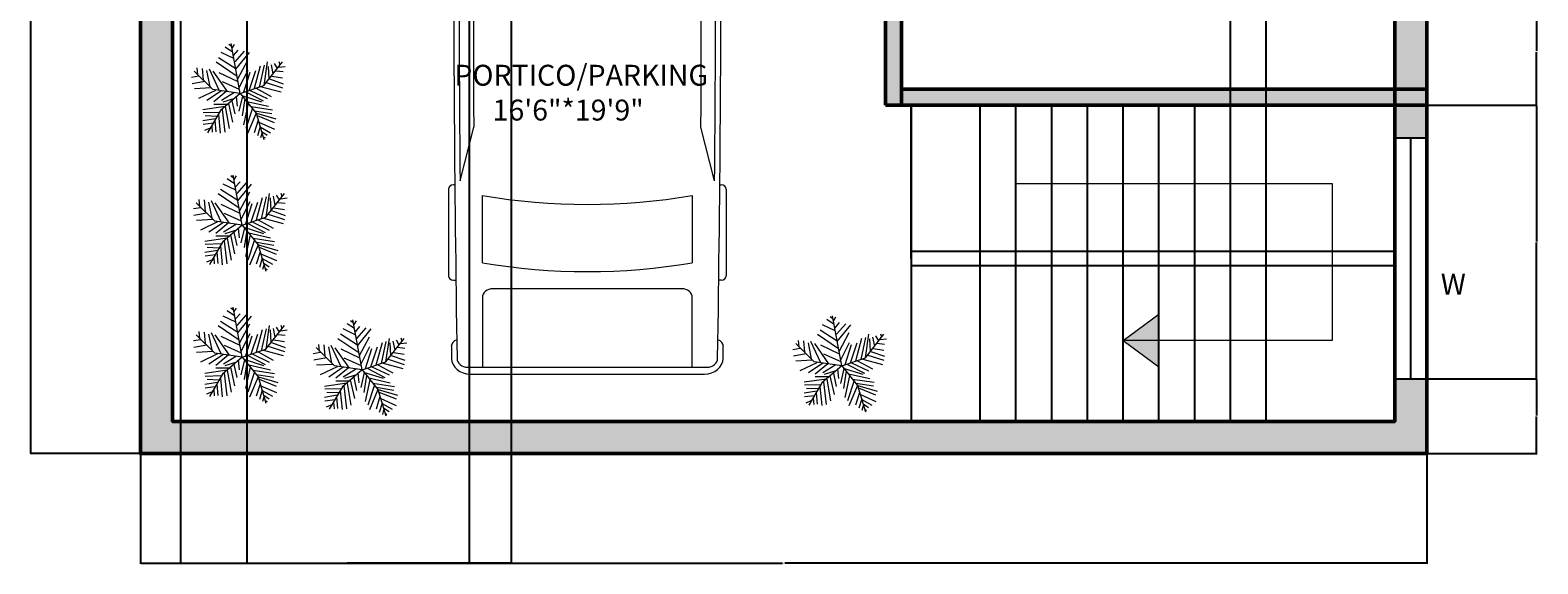
# Model space of a CAD drawing. Units: inches. Extents: x 678 to 1100, y 1432 to 2094.
# Tile 1 of 5: x 678 to 1100, y 1432 to 1581. Entities that reach past the tile are written whole.
import ezdxf

# ---------------------------------------------------------------- set-up
doc = ezdxf.new("R2010")
doc.units = ezdxf.units.IN
for name, color, linetype, lineweight in [('A-ANNO-DIMS', 2, 'Continuous', 18), ('A-ANNO-SYMB', 141, 'Continuous', 18), ('A-AREA-IDEN', 141, 'Continuous', 25), ('A-FLOR-STRS', 8, 'Continuous', 25), ('A-WALL-PATT', 252, 'Continuous', 13), ('C-PRKG-VEHI', 8, 'Continuous', 13), ('TEXT', 141, 'Continuous', 18), ('TREE', 90, 'Continuous', 13), ('WALL', 140, 'Continuous', 50), ('WIND', 212, 'Continuous', 25)]:
    doc.layers.add(name, color=color, linetype=linetype, lineweight=lineweight)
doc.styles.get("Standard").update_dxf_attribs({"font": 'arial.ttf'})
doc.dimstyles.get("Standard").update_dxf_attribs({"dimtxt": 0.18, "dimasz": 0.18, "dimexe": 0.18, "dimexo": 0.0625, "dimgap": 0.09, "dimtad": 0, "dimtih": 1, "dimtoh": 1, "dimdec": 4, "dimzin": 0, "dimdsep": 46, "dimtxsty": 'Standard', "dimcen": 0.09, "dimadec": 0, "dimazin": 0, "dimtfac": 1, "dimtdec": 4, "dimtofl": 0, "dimtmove": 0, "dimatfit": 3, "dimfxl": 1, "dimtolj": 1, "dimtzin": 0, "dimarcsym": 0})

# ---------------------------------------------------------------- blocks, each defined once
blk = doc.blocks.new('*U8')
for p, q in [((46.55, 38.89), (22.35, 38.89)), ((136.7, 38.89), (160.9, 38.89)), ((21.1, 37.41), (21.1, 36.83)), ((47.8, 37.39), (47.8, 37.41)), ((87.99, 31.87), (74.76, 35.92)), ((134.31, 35.6), (119.29, 31.78)), ((135.45, 37.07), (135.45, 37.41)), ((162.15, 37.41), (162.15, 36.77)), ((70.03, 31.54), (86.41, 29.35)), ((186.47, -33.5), (186.47, 33.5)), ((188.4, -32.76), (188.4, 32.76)), ((138.42, 29.35), (157.25, 29.35)), ((164.52, 26.39), (164.52, -26.39)), ((186.47, 29.35), (167.01, 29.35)), ((32.27, 11.63), (36.13, 17.17)), ((36.13, 17.17), (50.94, 17.17)), ((29.77, 9.51), (51.68, 9.51)), ((32.12, 9.51), (32.12, 11.15)), ((58.92, -10.77), (58.92, 10.77)), ((66.55, -10.53), (66.55, 10.53)), ((82.74, 8.5), (82.74, -8.5)), ((186.47, -10.53), (186.47, 10.53)), ((3.27, 6.13), (0.1, 0.41)), ((0, 0), (51.68, 0)), ((0.1, -0.41), (3.27, -6.13)), ((29.77, -9.51), (51.68, -9.51)), ((32.12, -9.51), (32.12, -11.15)), ((32.27, -11.63), (36.13, -17.17)), ((36.13, -17.17), (50.94, -17.17)), ((86.41, -29.35), (70.03, -31.54)), ((157.25, -29.35), (138.42, -29.35)), ((167.01, -29.35), (186.47, -29.35)), ((87.99, -31.87), (74.76, -35.92)), ((134.31, -35.6), (119.29, -31.78)), ((21.1, -37.41), (21.1, -36.83)), ((47.8, -37.39), (47.8, -37.41)), ((135.45, -37.07), (135.45, -37.41)), ((162.15, -37.41), (162.15, -36.77)), ((46.55, -38.89), (22.35, -38.89)), ((136.7, -38.89), (160.9, -38.89))]:
    blk.add_line(p, q)
for centre, major_axis, ratio, start_param, end_param in [((22.35, 37.41), (0, -1.48), 0.842304, 3.141593, 4.712389), ((46.55, 37.41), (0, 1.48), 0.842304, -1.570796, 0), ((136.7, 37.41), (0, -1.48), 0.842304, 3.141593, 4.712389), ((160.9, 37.41), (0, 1.48), 0.842304, -1.570796, 0), ((180.63, 35.84), (0, 2.22), 0.842304, -0.013017, 1.249894), ((64.48, -10556.36), (0, 10595.31), 0.842304, -0.013397, -0.013017), ((183.98, 32.76), (0, -5.25), 0.842304, 1.570796, 3.128196), ((266.03, -27.52), (0, 313.31), 0.842304, 1.367076, 1.39176), ((41.19, -490.86), (0, 528.23), 0.842304, 0.00281, 0.075598), ((64.48, -10555.62), (0, 10593.03), 0.842304, -0.013397, 0.002797), ((64.48, -10555.62), (0, -10591.55), 0.842304, 3.133765, 3.140441), ((183.98, 33.5), (0, -2.96), 0.842304, 1.570796, 3.128196), ((37.47, -593.96), (0, -623.33), 0.842304, 3.096046, 3.200911), ((135.29, 5.39), (0, 81.77), 0.842304, 1.245306, 1.50788), ((95.79, -3666.35), (0, -3698.24), 0.842304, 3.134049, 3.144098), ((259.18, -27.52), (0, -305.3), 0.842304, 4.528606, 4.561838), ((134.4, 5.39), (0, -89.78), 0.842304, 4.449482, 4.652344), ((149.6, 2.8), (0, -79.58), 0.842304, 4.372215, 4.640744), ((17.08, 0), (0, 147.02), 0.842304, 4.511394, 4.913384), ((35.91, 0), (0, 147.02), 0.842304, 4.511394, 4.913384), ((167.01, 26.39), (0, 2.96), 0.842304, 0, 1.570796), ((-204.49, 52.4), (0, -250.96), 0.842304, 1.385369, 1.434372), ((13.04, 17.01), (0, 27.42), 0.842304, 4.435146, 4.718221), ((14.2, 17.01), (0, 27.42), 0.842304, 4.435146, 4.718221), ((50.79, 13.34), (6.34, -0.36), 0.603834, -1.395552, 1.581315), ((29.77, -46.66), (0, 56.17), 0.842304, 0, 0.590319), ((32.75, 11.15), (0, 0.74), 0.842304, 0.879714, 1.570796), ((0.62, 0), (0, -0.74), 0.842304, 4.131459, 5.293319), ((29.77, 46.66), (0, 56.17), 0.842304, 2.551274, 3.141593), ((-204.49, -52.4), (0, 250.96), 0.842304, -1.434372, -1.385369), ((32.75, -11.15), (0, -0.74), 0.842304, 4.712389, 5.403472), ((13.04, -17.01), (0, -27.42), 0.842304, 1.564964, 1.848039), ((14.2, -17.01), (0, -27.42), 0.842304, 1.564964, 1.848039), ((134.4, -5.39), (0, -89.78), 0.842304, -1.510751, -1.307889), ((135.29, -5.39), (0, -81.77), 0.842304, -1.50788, -1.245306), ((149.6, -2.8), (0, -79.58), 0.842304, -1.499151, -1.230623), ((259.18, 27.52), (0, 305.3), 0.842304, 1.721348, 1.754579), ((266.03, 27.52), (0, 313.31), 0.842304, 1.749832, 1.774517), ((37.47, 593.96), (0, -623.33), 0.842304, -0.059319, 0.045547), ((167.01, -26.39), (0, -2.96), 0.842304, 4.712389, 6.283185), ((95.79, 3666.35), (0, -3698.24), 0.842304, -0.002505, 0.007544), ((183.98, -33.5), (0, 2.96), 0.842304, 3.15499, 4.712389), ((183.98, -32.76), (0, -5.25), 0.842304, 0.013397, 1.570796), ((41.19, 490.86), (0, -528.23), 0.842304, -0.075598, -0.00281), ((22.35, -37.41), (0, 1.48), 0.842304, 1.570796, 3.141593), ((64.48, 10555.62), (0, 10593.03), 0.842304, 3.138796, 3.15499), ((46.55, -37.41), (0, -1.48), 0.842304, 0, 1.570796), ((64.48, 10555.62), (0, -10591.55), 0.842304, 0.001152, 0.007828), ((136.7, -37.41), (0, -1.48), 0.842304, -1.570796, 0), ((160.9, -37.41), (0, 1.48), 0.842304, 3.141593, 4.712389), ((180.63, -35.84), (0, -2.22), 0.842304, -1.249894, 0.013017), ((64.48, 10556.36), (0, 10595.31), 0.842304, 3.15461, 3.15499)]:
    blk.add_ellipse(centre, major_axis=major_axis, ratio=ratio, start_param=start_param, end_param=end_param)
at = {"extrusion": (0, 0, -1)}
blk.add_ellipse((50.79, -13.34), major_axis=(6.34, 0.36), ratio=0.603834, start_param=-1.395552, end_param=1.581315, dxfattribs=at)
blk = doc.blocks.new('*U6')
for p, q in [((-8.737, 47.138), (-17.069, 52.711)), ((-10.186, 53.64), (-13.084, 55.962)), ((0, 0), (-10.5, 57)), ((-9.099, 51.782), (-6.563, 55.962)), ((-3.665, 19.273), (-27.574, 35.527)), ((-5.114, 28.097), (-24.676, 40.636)), ((-7.288, 39.707), (-21.778, 46.673)), ((-7.65, 43.423), (-2.578, 49.46)), ((-5.839, 35.992), (4.667, 48.067)), ((-5.114, 27.632), (10.463, 46.673)), ((-2.941, 16.486), (8.652, 37.85)), ((27, 9), (48, 36)), ((27.127, 9.056), (31.112, 35.992)), ((44.153, 36.456), (45.239, 32.741)), ((-47.498, 19.737), (-55.83, 18.344)), ((-31.5, 4.5), (-52.5, 25.5)), ((-48.585, 21.131), (-49.309, 29.026)), ((-43.513, 28.561), (-42.427, 15.558)), ((-38.442, 26.239), (-34.819, 7.663)), ((-35.544, 28.097), (-24.314, 3.947)), ((-14.533, 2.09), (-30.834, 25.31)), ((-24.314, 23.917), (-2.941, 13.7)), ((-1.129, 6.734), (9.014, 26.704)), ((3.942, 1.625), (11.187, 24.381)), ((10.101, 3.483), (17.708, 26.239)), ((16.259, 5.805), (23.142, 31.348)), ((22.055, 7.198), (27.489, 32.277)), ((31.836, 30.883), (32.561, 16.486)), ((35.096, 32.741), (37.27, 22.524)), ((36.183, 19.737), (48.137, 17.88)), ((38.719, 34.134), (41.979, 28.561)), ((40.53, 25.775), (48.862, 24.846)), ((43.791, 29.954), (51.036, 30.883)), ((-40.615, 13.7), (-55.105, 10.913)), ((-33.37, 6.269), (-52.207, 5.34)), ((-28.299, 3.483), (-47.86, -5.805)), ((-21.416, 3.018), (-38.079, -8.128)), ((0, 0), (-31.5, 4.5)), ((-15.982, 2.09), (-30.11, -9.521)), ((0, 0), (-22.5, -19.5)), ((-6.563, 1.161), (-21.416, -8.128)), ((-20.691, 13.7), (-1.129, 4.876)), ((0, 0), (27, 9)), ((0, 0), (18, -22.5)), ((6.478, 1.625), (26.04, -8.592)), ((11.187, 3.483), (30.749, -5.805)), ((18.07, 5.805), (35.096, -3.483)), ((24.229, 7.663), (46.688, 1.625)), ((29.662, 12.307), (48.137, 6.269)), ((33.285, 16.486), (48.862, 10.913)), ((-17.431, -15.094), (-42.789, -18.809)), ((-15.257, -12.772), (-30.11, -12.772)), ((-6.563, -5.805), (-19.967, -9.985)), ((-17.069, -15.094), (-12.721, -40.172)), ((-13.446, -11.378), (-8.737, -32.741)), ((-9.461, -8.592), (-6.201, -23.453)), ((-4.752, -3.483), (-3.665, -14.629)), ((2.493, -3.019), (-1.491, -20.202)), ((1.769, -2.555), (24.229, -9.521)), ((5.029, -6.27), (2.131, -25.775)), ((9.014, -11.378), (3.58, -35.992)), ((14.085, -16.951), (6.478, -40.172)), ((7.565, -9.056), (32.198, -14.629)), ((12.274, -15.094), (36.907, -18.809)), ((-28.299, -29.026), (-42.789, -31.348)), ((-24.314, -21.596), (-42.427, -22.06)), ((-30.834, -34.135), (-42.427, -35.528)), ((-26.849, -26.24), (-40.253, -25.775)), ((-22.5, -19.5), (-37.5, -45)), ((-29.023, -30.884), (-27.936, -43.887)), ((-25.038, -23.918), (-22.865, -45.281)), ((-20.691, -18.345), (-17.793, -44.352)), ((18.07, -22.524), (8.289, -45.745)), ((20.244, -30.419), (15.897, -44.816)), ((16.259, -19.738), (36.183, -22.989)), ((18, -22.5), (27, -52.5)), ((18.433, -22.524), (40.53, -29.026)), ((19.157, -25.311), (38.719, -33.206)), ((21.331, -32.741), (39.081, -40.636)), ((-34.457, -39.708), (-40.978, -42.494)), ((-32.646, -36.921), (-31.921, -44.352)), ((22.78, -37.85), (19.519, -48.532)), ((22.78, -38.314), (34.372, -44.816)), ((24.591, -45.745), (23.142, -50.854)), ((24.591, -43.423), (30.749, -47.603)), ((26.764, -49.925), (28.213, -50.854))]:
    blk.add_line(p, q)
blk = doc.blocks.new('WIN-STANDARD')
blk.add_line((4.5, 0), (4.5, 67.31))
blk.add_lwpolyline([(9, 67.31), (0, 67.31), (0, 0), (9, 0)], close=True)
blk = doc.blocks.new('*D24')
at = {"layer": 'A-ANNO-DIMS', "color": 0, "lineweight": -2, "transparency": 16777216}
for p, q in [((708.96, 1462.87), (708.96, 1432.1)), ((1068.96, 1462.87), (1068.96, 1432.1)), ((709.14, 1432.28), (888.67, 1432.28)), ((1068.78, 1432.28), (889.25, 1432.28))]:
    blk.add_line(p, q, dxfattribs=at)
at = {"layer": 'A-ANNO-DIMS', "color": 0, "transparency": 16777216}
for points in [[(709.14, 1432.31), (709.14, 1432.25), (708.96, 1432.28)], [(1068.78, 1432.31), (1068.78, 1432.25), (1068.96, 1432.28)]]:
    blk.add_solid(points, dxfattribs=at)
at = {"layer": 'Defpoints', "color": 0, "transparency": 16777216}
for p in [(708.96, 1462.93), (1068.96, 1462.93), (1068.96, 1432.28)]:
    blk.add_point(p, dxfattribs=at)
at = {"layer": 'A-ANNO-DIMS', "color": 0, "transparency": 16777216, "insert": (888.96, 1432.28), "char_height": 0.18, "attachment_point": 5}
blk.add_mtext('\\A1;360', dxfattribs=at)
blk = doc.blocks.new('*D25')
at = {"layer": 'A-ANNO-DIMS', "color": 0, "lineweight": -2, "transparency": 16777216}
for p, q in [((708.9, 2062.93), (678.13, 2062.93)), ((678.31, 2062.75), (678.31, 1763.11)), ((678.31, 1463.11), (678.31, 1762.75)), ((708.9, 1462.93), (678.13, 1462.93))]:
    blk.add_line(p, q, dxfattribs=at)
at = {"layer": 'A-ANNO-DIMS', "color": 0, "transparency": 16777216}
for points in [[(678.28, 2062.75), (678.34, 2062.75), (678.31, 2062.93)], [(678.28, 1463.11), (678.34, 1463.11), (678.31, 1462.93)]]:
    blk.add_solid(points, dxfattribs=at)
at = {"layer": 'Defpoints', "color": 0, "transparency": 16777216}
for p in [(678.31, 2062.93), (708.96, 2062.93), (708.96, 1462.93)]:
    blk.add_point(p, dxfattribs=at)
at = {"layer": 'A-ANNO-DIMS', "color": 0, "transparency": 16777216, "insert": (678.31, 1762.93), "char_height": 0.18, "attachment_point": 5}
blk.add_mtext('\\A1;600', dxfattribs=at)
blk = doc.blocks.new('*D31')
at = {"layer": 'A-ANNO-DIMS', "color": 0, "lineweight": -2, "transparency": 16777216}
for p, q in [((1069.02, 1483.85), (1099.79, 1483.85)), ((1099.61, 1483.67), (1099.61, 1473.57)), ((1099.61, 1463.11), (1099.61, 1473.21)), ((1069.02, 1462.93), (1099.79, 1462.93))]:
    blk.add_line(p, q, dxfattribs=at)
at = {"layer": 'A-ANNO-DIMS', "color": 0, "transparency": 16777216}
for points in [[(1099.58, 1483.67), (1099.64, 1483.67), (1099.61, 1483.85)], [(1099.58, 1463.11), (1099.64, 1463.11), (1099.61, 1462.93)]]:
    blk.add_solid(points, dxfattribs=at)
at = {"layer": 'Defpoints', "color": 0, "transparency": 16777216}
for p in [(1068.96, 1483.85), (1099.61, 1483.85), (1068.96, 1462.93)]:
    blk.add_point(p, dxfattribs=at)
at = {"layer": 'A-ANNO-DIMS', "color": 0, "transparency": 16777216, "insert": (1099.61, 1473.39), "char_height": 0.18, "attachment_point": 5}
blk.add_mtext('\\A1;20.922', dxfattribs=at)
blk = doc.blocks.new('*D32')
at = {"layer": 'A-ANNO-DIMS', "color": 0, "lineweight": -2, "transparency": 16777216}
for p, q in [((1069.02, 1560.43), (1099.79, 1560.43)), ((1099.61, 1560.25), (1099.61, 1522.32)), ((1099.61, 1484.03), (1099.61, 1521.96)), ((1069.02, 1483.85), (1099.79, 1483.85))]:
    blk.add_line(p, q, dxfattribs=at)
at = {"layer": 'A-ANNO-DIMS', "color": 0, "transparency": 16777216}
for points in [[(1099.58, 1560.25), (1099.64, 1560.25), (1099.61, 1560.43)], [(1099.58, 1484.03), (1099.64, 1484.03), (1099.61, 1483.85)]]:
    blk.add_solid(points, dxfattribs=at)
at = {"layer": 'Defpoints', "color": 0, "transparency": 16777216}
for p in [(1068.96, 1560.43), (1099.61, 1560.43), (1068.96, 1483.85)]:
    blk.add_point(p, dxfattribs=at)
at = {"layer": 'A-ANNO-DIMS', "color": 0, "transparency": 16777216, "insert": (1099.61, 1522.14), "char_height": 0.18, "attachment_point": 5}
blk.add_mtext('\\A1;76.58', dxfattribs=at)
blk = doc.blocks.new('*D33')
at = {"layer": 'A-ANNO-DIMS', "color": 0, "lineweight": -2, "transparency": 16777216}
for p, q in [((1069.02, 1590.39), (1099.79, 1590.39)), ((1099.61, 1590.21), (1099.61, 1575.59)), ((1099.61, 1560.61), (1099.61, 1575.23)), ((1069.02, 1560.43), (1099.79, 1560.43))]:
    blk.add_line(p, q, dxfattribs=at)
at = {"layer": 'A-ANNO-DIMS', "color": 0, "transparency": 16777216}
for points in [[(1099.58, 1590.21), (1099.64, 1590.21), (1099.61, 1590.39)], [(1099.58, 1560.61), (1099.64, 1560.61), (1099.61, 1560.43)]]:
    blk.add_solid(points, dxfattribs=at)
at = {"layer": 'Defpoints', "color": 0, "transparency": 16777216}
for p in [(1068.96, 1590.39), (1099.61, 1590.39), (1068.96, 1560.43)]:
    blk.add_point(p, dxfattribs=at)
at = {"layer": 'A-ANNO-DIMS', "color": 0, "transparency": 16777216, "insert": (1099.61, 1575.41), "char_height": 0.18, "attachment_point": 5}
blk.add_mtext('\\A1;29.96', dxfattribs=at)
blk = doc.blocks.new('*D48')
at = {"layer": 'A-ANNO-DIMS', "color": 0, "lineweight": -2, "transparency": 16777216}
for p, q in [((917.46, 1560.49), (917.46, 2093.76)), ((917.64, 2093.58), (919.45, 2093.58)), ((921.78, 2093.58), (919.97, 2093.58)), ((921.96, 1560.49), (921.96, 2093.76))]:
    blk.add_line(p, q, dxfattribs=at)
at = {"layer": 'A-ANNO-DIMS', "color": 0, "transparency": 16777216}
for points in [[(917.64, 2093.61), (917.64, 2093.55), (917.46, 2093.58)], [(921.78, 2093.61), (921.78, 2093.55), (921.96, 2093.58)]]:
    blk.add_solid(points, dxfattribs=at)
at = {"layer": 'Defpoints', "color": 0, "transparency": 16777216}
for p in [(921.96, 2093.58), (917.46, 1560.43), (921.96, 1560.43)]:
    blk.add_point(p, dxfattribs=at)
at = {"layer": 'A-ANNO-DIMS', "color": 0, "transparency": 16777216, "insert": (919.71, 2093.58), "char_height": 0.18, "attachment_point": 5}
blk.add_mtext('\\A1;4.5', dxfattribs=at)
blk = doc.blocks.new('*D49')
at = {"layer": 'A-ANNO-DIMS', "color": 0, "lineweight": -2, "transparency": 16777216}
for p, q in [((1013.96, 1471.99), (1013.96, 2093.76)), ((1014.14, 2093.58), (1018.75, 2093.58)), ((1023.78, 2093.58), (1019.17, 2093.58)), ((1023.96, 1471.99), (1023.96, 2093.76))]:
    blk.add_line(p, q, dxfattribs=at)
at = {"layer": 'A-ANNO-DIMS', "color": 0, "transparency": 16777216}
for points in [[(1014.14, 2093.61), (1014.14, 2093.55), (1013.96, 2093.58)], [(1023.78, 2093.61), (1023.78, 2093.55), (1023.96, 2093.58)]]:
    blk.add_solid(points, dxfattribs=at)
at = {"layer": 'Defpoints', "color": 0, "transparency": 16777216}
for p in [(1023.96, 2093.58), (1013.96, 1471.93), (1023.96, 1471.93)]:
    blk.add_point(p, dxfattribs=at)
at = {"layer": 'A-ANNO-DIMS', "color": 0, "transparency": 16777216, "insert": (1018.96, 2093.58), "char_height": 0.18, "attachment_point": 5}
blk.add_mtext('\\A1;10', dxfattribs=at)
blk = doc.blocks.new('*D50')
at = {"layer": 'A-ANNO-DIMS', "color": 0, "lineweight": -2, "transparency": 16777216}
for p, q in [((1023.96, 1471.99), (1023.96, 2093.76)), ((1024.14, 2093.58), (1041.74, 2093.58)), ((1059.78, 2093.58), (1042.18, 2093.58)), ((1059.96, 1471.99), (1059.96, 2093.76))]:
    blk.add_line(p, q, dxfattribs=at)
at = {"layer": 'A-ANNO-DIMS', "color": 0, "transparency": 16777216}
for points in [[(1024.14, 2093.61), (1024.14, 2093.55), (1023.96, 2093.58)], [(1059.78, 2093.61), (1059.78, 2093.55), (1059.96, 2093.58)]]:
    blk.add_solid(points, dxfattribs=at)
at = {"layer": 'Defpoints', "color": 0, "transparency": 16777216}
for p in [(1059.96, 2093.58), (1023.96, 1471.93), (1059.96, 1471.93)]:
    blk.add_point(p, dxfattribs=at)
at = {"layer": 'A-ANNO-DIMS', "color": 0, "transparency": 16777216, "insert": (1041.96, 2093.58), "char_height": 0.18, "attachment_point": 5}
blk.add_mtext('\\A1;36', dxfattribs=at)
blk = doc.blocks.new('*D53')
at = {"layer": 'A-ANNO-DIMS', "color": 0, "lineweight": -2, "transparency": 16777216}
for p, q in [((738.71, 1897.06), (738.71, 1432.1)), ((800.95, 1897.06), (800.95, 1432.1)), ((738.89, 1432.28), (769.43, 1432.28)), ((800.77, 1432.28), (770.22, 1432.28))]:
    blk.add_line(p, q, dxfattribs=at)
at = {"layer": 'A-ANNO-DIMS', "color": 0, "transparency": 16777216}
for points in [[(738.89, 1432.31), (738.89, 1432.25), (738.71, 1432.28)], [(800.77, 1432.31), (800.77, 1432.25), (800.95, 1432.28)]]:
    blk.add_solid(points, dxfattribs=at)
at = {"layer": 'Defpoints', "color": 0, "transparency": 16777216}
for p in [(738.71, 1897.12), (800.95, 1897.12), (800.95, 1432.28)]:
    blk.add_point(p, dxfattribs=at)
at = {"layer": 'A-ANNO-DIMS', "color": 0, "transparency": 16777216, "insert": (769.83, 1432.28), "char_height": 0.18, "attachment_point": 5}
blk.add_mtext('\\A1;62.25', dxfattribs=at)
blk = doc.blocks.new('*D55')
at = {"layer": 'A-ANNO-DIMS', "color": 0, "lineweight": -2, "transparency": 16777216}
for p, q in [((812.72, 1833.21), (812.72, 1432.1)), ((720.22, 1787.87), (720.22, 1432.1)), ((720.4, 1432.28), (766.15, 1432.28)), ((812.54, 1432.28), (766.8, 1432.28))]:
    blk.add_line(p, q, dxfattribs=at)
at = {"layer": 'A-ANNO-DIMS', "color": 0, "transparency": 16777216}
for points in [[(720.4, 1432.31), (720.4, 1432.25), (720.22, 1432.28)], [(812.54, 1432.31), (812.54, 1432.25), (812.72, 1432.28)]]:
    blk.add_solid(points, dxfattribs=at)
at = {"layer": 'Defpoints', "color": 0, "transparency": 16777216}
for p in [(812.72, 1833.27), (720.22, 1787.94), (812.72, 1432.28)]:
    blk.add_point(p, dxfattribs=at)
at = {"layer": 'A-ANNO-DIMS', "color": 0, "transparency": 16777216, "insert": (766.47, 1432.28), "char_height": 0.18, "attachment_point": 5}
blk.add_mtext('\\A1;92.5', dxfattribs=at)

msp = doc.modelspace()

# ---------------------------------------------------------------- hatches: boundary and pattern name
at = {"layer": 'A-ANNO-SYMB'}
h = msp.add_hatch(color=256, dxfattribs=at)
h.dxf.hatch_style = 1
h.paths.add_polyline_path([(993.9606, 1501.9868), (983.9606, 1494.6187), (993.9606, 1494.6187)])
h.paths.add_polyline_path([(993.9606, 1494.6187), (983.9606, 1494.6187), (993.9606, 1487.2506)])
at = {"layer": 'A-WALL-PATT'}
h = msp.add_hatch(color=256, dxfattribs=at)
h.dxf.hatch_style = 1
h.paths.add_polyline_path([(859.7133, 2062.9286), (708.9606, 2062.9286), (708.9606, 2031.3203), (717.9606, 2031.3203), (717.9606, 2053.9286), (837.9606, 2053.9286), (859.7133, 2053.9286)])
h.paths.add_polyline_path([(957.0069, 2062.9286), (896.0724, 2062.9286), (896.0724, 2053.9286), (957.0069, 2053.9286)])
h.paths.add_polyline_path([(842.4606, 2053.9286), (837.9606, 2053.9286), (837.9606, 2005.4286), (842.4606, 2005.4286), (923.4606, 2005.4286), (923.4606, 2009.9286), (842.4606, 2009.9286)])
h.paths.add_polyline_path([(927.9606, 2053.9286), (923.4606, 2053.9286), (923.4606, 2052.1286), (924.8103, 2052.1286), (927.9606, 2052.1286)])
h.paths.add_polyline_path([(1068.9606, 2062.9286), (1024.3184, 2062.9286), (1024.3184, 2053.9286), (1028.6041, 2053.9286), (1059.9606, 2053.9286), (1059.9606, 2002.6361), (1068.9606, 2002.6361)])
h.paths.add_polyline_path([(1059.9606, 1861.9286), (996.9604, 1861.9286), (927.9606, 1861.9286), (923.4606, 1861.9286), (923.4606, 1857.4286), (1059.9606, 1857.4286)], flags=17)
h.paths.add_polyline_path([(927.9606, 2031.1269), (924.8103, 2031.1269, -0.01607952), (923.4606, 2031.1703), (923.4606, 1905.3856), (927.9606, 1905.3856)])
h.paths.add_polyline_path([(923.4606, 1957.9286), (842.4606, 1957.9286), (842.4606, 1969.339), (837.9606, 1969.339), (837.9606, 1953.4286), (923.4606, 1953.4286)])
h.paths.add_polyline_path([(774.6357, 1957.9286), (717.9606, 1957.9286), (717.9606, 1953.4286), (774.6357, 1953.4286)])
h.paths.add_polyline_path([(717.9606, 1979.9404), (708.9606, 1979.9404), (708.9606, 1945.1463), (717.9606, 1945.1463)])
h.paths.add_polyline_path([(840.5596, 1861.9286), (717.9606, 1861.9286), (717.9606, 1857.4286), (840.5596, 1857.4286)], flags=17)
h.paths.add_polyline_path([(927.9606, 1865.3856), (923.4606, 1865.3856), (923.4606, 1861.9286), (927.9606, 1861.9286)], flags=17)
h.paths.add_polyline_path([(1059.9606, 1689.4286), (967.3461, 1689.4286), (967.3461, 1684.9286), (1059.9606, 1684.9286)], flags=17)
h.paths.add_polyline_path([(987.9606, 1737.4286), (983.4606, 1737.4286), (983.4606, 1715.196), (986.7357, 1715.196, -0.01403382), (987.9606, 1715.1616)], flags=17)
h.paths.add_polyline_path([(916.0499, 2036.8414), (924.8721, 2036.8414), (924.8721, 2048.8901), (916.0499, 2048.8901)], flags=9)
h.paths.add_polyline_path([(921.7778, 1883.2914), (930.5999, 1883.2914), (930.5999, 1895.3401), (921.7778, 1895.3401)], flags=25)
h.paths.add_polyline_path([(732.1085, 1683.0506), (740.9307, 1683.0506), (740.9307, 1695.0993), (732.1085, 1695.0993)], flags=25)
h.paths.add_polyline_path([(943.8458, 1737.5114), (952.6679, 1737.5114), (952.6679, 1749.5601), (943.8458, 1749.5601)], flags=25)
h.paths.add_polyline_path([(986.0751, 1696.9795), (994.8973, 1696.9795), (994.8973, 1709.0282), (986.0751, 1709.0282)], flags=25)
h.paths.add_polyline_path([(940.1881, 1677.378), (949.0103, 1677.378), (949.0103, 1689.4267), (940.1881, 1689.4267)], flags=25)
h.paths.add_polyline_path([(998.6262, 1761.7469), (1044.0453, 1761.7469), (1044.0453, 1783.5644), (998.6262, 1783.5644)], flags=25)
h.paths.add_polyline_path([(997.3001, 1713.4735), (1028.9316, 1713.4735), (1028.9316, 1735.2909), (997.3001, 1735.2909)], flags=25)
h.paths.add_polyline_path([(1005.9896, 1586.8139), (1051.4087, 1586.8139), (1051.4087, 1608.6313), (1005.9896, 1608.6313)], flags=25)
h.paths.add_polyline_path([(794.7038, 1552.8124), (873.8721, 1552.8124), (873.8721, 1574.6298), (794.7038, 1574.6298)], flags=25)
h.paths.add_polyline_path([(774.2693, 1771.1228), (831.9444, 1771.1228), (831.9444, 1792.9403), (774.2693, 1792.9403)], flags=25)
h.paths.add_polyline_path([(750.0357, 1897.1514), (786.4291, 1897.1514), (786.4291, 1918.9689), (750.0357, 1918.9689)], flags=25)
h.paths.add_polyline_path([(974.9086, 1953.7921), (1020.3276, 1953.7921), (1020.3276, 1975.6096), (974.9086, 1975.6096)], flags=9)
h.paths.add_polyline_path([(859.1564, 1973.8092), (890.2175, 1973.8092), (890.2175, 1995.6267), (859.1564, 1995.6267)], flags=9)
h.paths.add_polyline_path([(753.2305, 1989.0219), (792.2962, 1989.0219), (792.2962, 2010.8393), (753.2305, 2010.8393)], flags=9)
h.paths.add_polyline_path([(1067.3992, 1620.1515), (1078.032, 1620.1515), (1078.032, 1632.2002), (1067.3992, 1632.2002)], flags=9)
h.paths.add_polyline_path([(846.8446, 2028.8178), (878.5079, 2028.8178), (878.5079, 2050.6353), (846.8446, 2050.6353)], flags=25)
h.paths.add_polyline_path([(1059.9606, 1832.7202), (1068.9606, 1832.7202), (1068.9606, 1935.3246), (1059.9606, 1935.3246)])
h.paths.add_polyline_path([(1068.9606, 1765.4088), (1059.9606, 1765.4088), (1059.9606, 1728.1446), (1068.9606, 1728.1446)])
h.paths.add_polyline_path([(1059.9606, 1657.7018), (1068.9606, 1657.7018), (1068.9606, 1697.8017), (1059.9606, 1697.8017)])
h.paths.add_polyline_path([(1068.9606, 1590.3903), (1059.9606, 1590.3903), (1059.9606, 1551.1623), (1068.9606, 1551.1623)])
h.paths.add_polyline_path([(708.9606, 1826.8331), (717.9606, 1826.8331), (717.9606, 1877.8348), (708.9606, 1877.8348)])
h.paths.add_polyline_path([(717.9606, 1759.5217), (708.9606, 1759.5217), (708.9606, 1462.9286), (1068.9606, 1462.9286), (1068.9606, 1483.8508), (1059.9606, 1483.8508), (1059.9606, 1471.9286), (717.9606, 1471.9286)])
h = msp.add_hatch(color=256, dxfattribs=at)
h.dxf.hatch_style = 1
h.paths.add_polyline_path([(1059.9606, 1741.9286), (970.7942, 1741.9286), (970.7942, 1737.4286), (1059.9606, 1737.4286)])
h.paths.add_polyline_path([(927.3461, 1689.4286), (759.4099, 1689.4286), (759.4099, 1684.9286), (927.3461, 1684.9286)])
h.paths.add_polyline_path([(921.9606, 1684.9286), (917.4606, 1684.9286), (917.4606, 1560.4286), (921.9606, 1560.4286)])
h.paths.add_polyline_path([(1059.9606, 1564.9286), (921.9606, 1564.9286), (921.9606, 1560.4286), (1059.9606, 1560.4286)])
h.paths.add_polyline_path([(916.0499, 2036.8414), (924.8721, 2036.8414), (924.8721, 2048.8901), (916.0499, 2048.8901)], flags=9)
h.paths.add_polyline_path([(921.7778, 1883.2914), (930.5999, 1883.2914), (930.5999, 1895.3401), (921.7778, 1895.3401)], flags=9)
h.paths.add_polyline_path([(732.1085, 1683.0506), (740.9307, 1683.0506), (740.9307, 1695.0993), (732.1085, 1695.0993)], flags=9)
h.paths.add_polyline_path([(943.8458, 1737.5114), (952.6679, 1737.5114), (952.6679, 1749.5601), (943.8458, 1749.5601)], flags=9)
h.paths.add_polyline_path([(986.0751, 1696.9795), (994.8973, 1696.9795), (994.8973, 1709.0282), (986.0751, 1709.0282)], flags=9)
h.paths.add_polyline_path([(940.1881, 1677.378), (949.0103, 1677.378), (949.0103, 1689.4267), (940.1881, 1689.4267)], flags=9)
h.paths.add_polyline_path([(998.6262, 1761.7469), (1044.0453, 1761.7469), (1044.0453, 1783.5644), (998.6262, 1783.5644)], flags=9)
h.paths.add_polyline_path([(1005.9896, 1586.8139), (1051.4087, 1586.8139), (1051.4087, 1608.6313), (1005.9896, 1608.6313)], flags=9)
h.paths.add_polyline_path([(794.7038, 1552.8124), (873.8721, 1552.8124), (873.8721, 1574.6298), (794.7038, 1574.6298)], flags=9)
h.paths.add_polyline_path([(774.2693, 1771.1228), (831.9444, 1771.1228), (831.9444, 1792.9403), (774.2693, 1792.9403)], flags=9)
h.paths.add_polyline_path([(750.0357, 1897.1514), (786.4291, 1897.1514), (786.4291, 1918.9689), (750.0357, 1918.9689)], flags=9)
h.paths.add_polyline_path([(974.9086, 1953.7921), (1020.3276, 1953.7921), (1020.3276, 1975.6096), (974.9086, 1975.6096)], flags=9)
h.paths.add_polyline_path([(859.1564, 1973.8092), (890.2175, 1973.8092), (890.2175, 1995.6267), (859.1564, 1995.6267)], flags=9)
h.paths.add_polyline_path([(846.8446, 2028.8178), (878.5079, 2028.8178), (878.5079, 2050.6353), (846.8446, 2050.6353)], flags=9)
h.paths.add_polyline_path([(753.2305, 1989.0219), (792.2962, 1989.0219), (792.2962, 2010.8393), (753.2305, 2010.8393)], flags=9)
h = msp.add_hatch(color=256, dxfattribs=at)
h.dxf.hatch_style = 1
h.paths.add_polyline_path([(927.9606, 1857.4286), (923.4606, 1857.4286), (923.4606, 1737.4286), (927.9606, 1737.4286)])
h.paths.add_polyline_path([(930.7942, 1741.9286), (927.9606, 1741.9286), (927.9606, 1737.4286), (930.7942, 1737.4286)])
h.paths.add_polyline_path([(916.0499, 2036.8414), (924.8721, 2036.8414), (924.8721, 2048.8901), (916.0499, 2048.8901)], flags=9)
h.paths.add_polyline_path([(921.7778, 1883.2914), (930.5999, 1883.2914), (930.5999, 1895.3401), (921.7778, 1895.3401)], flags=9)
h.paths.add_polyline_path([(732.1085, 1683.0506), (740.9307, 1683.0506), (740.9307, 1695.0993), (732.1085, 1695.0993)], flags=9)
h.paths.add_polyline_path([(943.8458, 1737.5114), (952.6679, 1737.5114), (952.6679, 1749.5601), (943.8458, 1749.5601)], flags=9)
h.paths.add_polyline_path([(986.0751, 1696.9795), (994.8973, 1696.9795), (994.8973, 1709.0282), (986.0751, 1709.0282)], flags=9)
h.paths.add_polyline_path([(940.1881, 1677.378), (949.0103, 1677.378), (949.0103, 1689.4267), (940.1881, 1689.4267)], flags=9)
h.paths.add_polyline_path([(998.6262, 1761.7469), (1044.0453, 1761.7469), (1044.0453, 1783.5644), (998.6262, 1783.5644)], flags=9)
h.paths.add_polyline_path([(997.3001, 1713.4735), (1028.9316, 1713.4735), (1028.9316, 1735.2909), (997.3001, 1735.2909)], flags=9)
h.paths.add_polyline_path([(1005.9896, 1586.8139), (1051.4087, 1586.8139), (1051.4087, 1608.6313), (1005.9896, 1608.6313)], flags=9)
h.paths.add_polyline_path([(794.7038, 1552.8124), (873.8721, 1552.8124), (873.8721, 1574.6298), (794.7038, 1574.6298)], flags=9)
h.paths.add_polyline_path([(774.2693, 1771.1228), (831.9444, 1771.1228), (831.9444, 1792.9403), (774.2693, 1792.9403)], flags=9)
h.paths.add_polyline_path([(750.0357, 1897.1514), (786.4291, 1897.1514), (786.4291, 1918.9689), (750.0357, 1918.9689)], flags=9)
h.paths.add_polyline_path([(974.9086, 1953.7921), (1020.3276, 1953.7921), (1020.3276, 1975.6096), (974.9086, 1975.6096)], flags=9)
h.paths.add_polyline_path([(859.1564, 1973.8092), (890.2175, 1973.8092), (890.2175, 1995.6267), (859.1564, 1995.6267)], flags=9)
h.paths.add_polyline_path([(846.8446, 2028.8178), (878.5079, 2028.8178), (878.5079, 2050.6353), (846.8446, 2050.6353)], flags=9)
h.paths.add_polyline_path([(753.2305, 1989.0219), (792.2962, 1989.0219), (792.2962, 2010.8393), (753.2305, 2010.8393)], flags=9)

# ---------------------------------------------------------------- linework, layer by layer
at = {"layer": 'A-ANNO-SYMB'}
for p, q in [((953.9606, 1538.5117), (1042.392, 1538.5117)), ((1042.392, 1538.5117), (1042.392, 1494.6187)), ((983.9606, 1494.6187), (993.9606, 1501.9868)), ((1042.392, 1494.6187), (983.9606, 1494.6187)), ((983.9606, 1494.6187), (993.9606, 1487.2506))]:
    msp.add_line(p, q, dxfattribs=at)
at = {"layer": 'A-FLOR-STRS'}
for p, q in [((924.5896, 1517.5066), (924.5896, 1560.4286)), ((924.5896, 1560.4286), (924.5896, 1471.9286)), ((943.9606, 1471.9286), (943.9606, 1560.4286)), ((953.9606, 1471.9286), (953.9606, 1560.4286)), ((963.9606, 1471.9286), (963.9606, 1560.4286)), ((973.9606, 1471.9286), (973.9606, 1560.4286)), ((983.9606, 1471.9286), (983.9606, 1560.4286)), ((993.9606, 1471.9286), (993.9606, 1560.4286)), ((1003.9606, 1471.9286), (1003.9606, 1560.4286)), ((1013.9606, 1471.9286), (1013.9606, 1560.4286)), ((1023.9606, 1471.9286), (1023.9606, 1560.4286)), ((1059.9606, 1519.5066), (924.5896, 1519.5066)), ((1059.9606, 1515.5066), (924.5896, 1515.5066))]:
    msp.add_line(p, q, dxfattribs=at)
at = {"layer": 'WALL'}
for p, q in [((708.9606, 1462.9286), (708.9606, 2062.9286)), ((1068.9606, 2062.9286), (1068.9606, 1462.9286)), ((717.9606, 1471.9286), (717.9606, 1708.9286)), ((917.4606, 1684.9286), (917.4606, 1560.4286)), ((921.9606, 1684.9286), (921.9606, 1564.9286)), ((921.9606, 1564.9286), (1068.9606, 1564.9286)), ((917.4606, 1560.4286), (1068.9606, 1560.4286)), ((717.9606, 1471.9286), (915.9606, 1471.9286)), ((1059.9606, 1471.9286), (1023.9606, 1471.9286)), ((1068.9606, 1462.9286), (708.9606, 1462.9286))]:
    msp.add_line(p, q, dxfattribs=at)
for points in [[(708.9606, 2062.9286), (1068.9606, 2062.9286), (1068.9606, 1462.9286), (708.9606, 1462.9286)], [(717.9606, 2053.9286), (1059.9606, 2053.9286), (1059.9606, 1471.9286), (717.9606, 1471.9286)], [(917.4606, 1560.4286), (921.9606, 1560.4286), (921.9606, 1684.9286), (917.4606, 1684.9286)], [(1059.9606, 1560.4286), (921.9606, 1560.4286), (921.9606, 1564.9286), (1059.9606, 1564.9286)]]:
    msp.add_lwpolyline(points, close=True, dxfattribs=at)

# ---------------------------------------------------------------- block references
at = {"layer": 'C-PRKG-VEHI', "rotation": 270}
msp.add_blockref('*U8', (834.016, 1673.5922), dxfattribs=at)
at = {"layer": 'TREE', "xscale": 0.2451816363405065, "yscale": 0.2451816363405065, "zscale": 0.2451816363405065}
for p in [(736.9048, 1563.717), (737.4639, 1526.8939), (737.4639, 1489.957), (770.9863, 1486.3639), (905.1944, 1487.5084)]:
    msp.add_blockref('*U6', p, dxfattribs=at)
at = {"layer": 'WIND'}
msp.add_blockref('WIN-STANDARD', (1059.961, 1483.851), dxfattribs=at)

# ---------------------------------------------------------------- texts
at = {"layer": 'A-AREA-IDEN', "insert": (796.7957, 1571.7243), "char_height": 5.846885, "attachment_point": 1}
msp.add_mtext_dynamic_manual_height_columns('PORTICO/PARKING\\P      16\'6"*19\'9"', width=180.890738, gutter_width=29.2344, heights=[0], dxfattribs=at)
at = {"layer": 'TEXT', "insert": (1072.8234, 1513.2591), "char_height": 5.8469, "attachment_point": 1}
msp.add_mtext_dynamic_manual_height_columns('W', width=180.890738, gutter_width=29.2344, heights=[0], dxfattribs=at)

# ---------------------------------------------------------------- dimensions: what is measured, and where the dimension line sits
at = {"layer": 'A-ANNO-DIMS'}
for base, p1, p2, override, picture, middle in [((921.9606, 2093.5786), (917.4606, 1560.4286), (921.9606, 1560.4286), {"dimdec": 1, "dimlfac": 1, "dimrnd": 0, "dimzin": 0, "dimdsep": 46, "dimlunit": 2}, '*D48', (919.7106, 2093.5786)), ((1023.9606, 2093.5786), (1013.9606, 1471.9286), (1023.9606, 1471.9286), {"dimdec": 0, "dimlfac": 1, "dimrnd": 0, "dimzin": 0, "dimdsep": 46, "dimlunit": 2}, '*D49', (1018.9606, 2093.5786)), ((1059.9606, 2093.5786), (1023.9606, 1471.9286), (1059.9606, 1471.9286), {"dimdec": 0, "dimlfac": 1, "dimrnd": 0, "dimzin": 0, "dimdsep": 46, "dimlunit": 2}, '*D50', (1041.9606, 2093.5786)), ((800.9505, 1432.2786), (738.7053, 1897.12), (800.9505, 1897.12), {"dimdec": 2, "dimlfac": 1, "dimrnd": 0, "dimzin": 0, "dimdsep": 46, "dimlunit": 2}, '*D53', (769.8279, 1432.2786)), ((812.7228, 1432.2786), (720.2201, 1787.9351), (812.7228, 1833.2731), {"dimdec": 1, "dimlfac": 1, "dimrnd": 0, "dimzin": 0, "dimdsep": 46, "dimlunit": 2}, '*D55', (766.4715, 1432.2786)), ((1068.9606, 1432.2786), (708.9606, 1462.9286), (1068.9606, 1462.9286), {"dimdec": 0, "dimlfac": 1, "dimrnd": 0, "dimzin": 0, "dimdsep": 46, "dimlunit": 2}, '*D24', (888.9606, 1432.2786))]:
    dim = msp.add_linear_dim(base=base, p1=p1, p2=p2, dimstyle='Standard', override=override, dxfattribs=at)
    dim.commit()
    dim.dimension.update_dxf_attribs({"geometry": picture, "text_midpoint": middle})
for base, p1, p2, override, picture, middle in [((678.3106, 2062.9286), (708.9606, 1462.9286), (708.9606, 2062.9286), {"dimdec": 0, "dimlfac": 1, "dimrnd": 0, "dimzin": 0, "dimdsep": 46, "dimlunit": 2}, '*D25', (678.3106, 1762.9286)), ((1099.6106, 1590.3903), (1068.9606, 1560.4286), (1068.9606, 1590.3903), {"dimdec": 2, "dimlfac": 1, "dimrnd": 0, "dimzin": 0, "dimdsep": 46, "dimlunit": 2}, '*D33', (1099.6106, 1575.4094)), ((1099.6106, 1560.4286), (1068.9606, 1483.8508), (1068.9606, 1560.4286), {"dimdec": 2, "dimlfac": 1, "dimrnd": 0, "dimzin": 0, "dimdsep": 46, "dimlunit": 2}, '*D32', (1099.6106, 1522.1397)), ((1099.6106, 1483.8508), (1068.9606, 1462.9286), (1068.9606, 1483.8508), {"dimdec": 3, "dimlfac": 1, "dimrnd": 0, "dimzin": 0, "dimdsep": 46, "dimlunit": 2}, '*D31', (1099.6106, 1473.3897))]:
    dim = msp.add_linear_dim(base=base, p1=p1, p2=p2, angle=90, dimstyle='Standard', override=override, dxfattribs=at)
    dim.commit()
    dim.dimension.update_dxf_attribs({"geometry": picture, "text_midpoint": middle})

doc.saveas('drawing.dxf')
